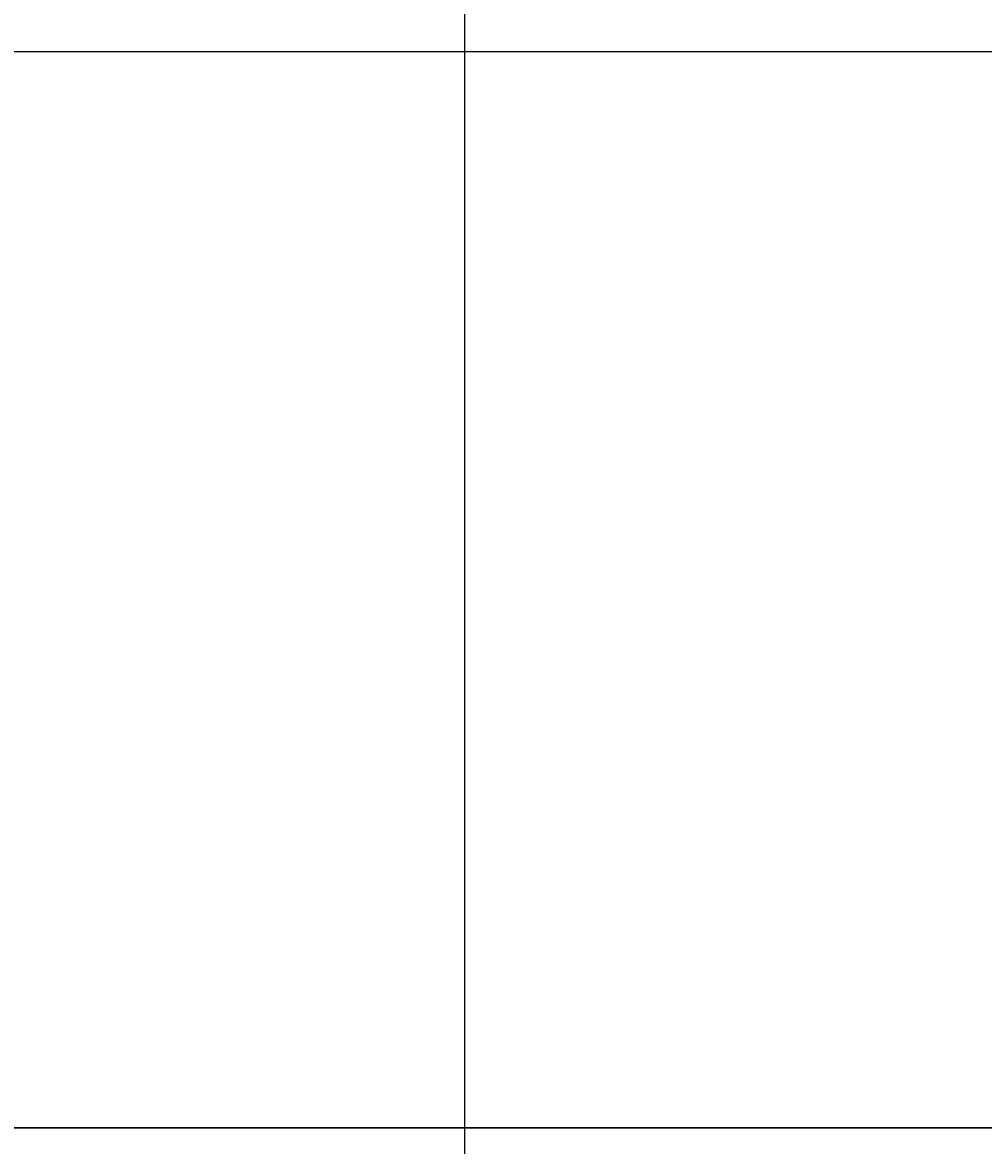
# Model space of a CAD drawing. Units: feet. Extents: x 105 to 1094, y -88 to 588.
# Tile 56 of 59: x 649 to 699, y 470 to 529. Entities that reach past the tile are written whole.
import ezdxf

# ---------------------------------------------------------------- set-up
doc = ezdxf.new("R2010")
doc.units = ezdxf.units.FT
doc.header["$MEASUREMENT"] = 0
doc.layers.add('A-ANNO-DIMS', color=2, linetype='Continuous', lineweight=18)
doc.layers.add('A-FLOR-PROJ', color=8, linetype='Continuous', lineweight=25)
doc.styles.get("Standard").update_dxf_attribs({"font": 'arial.ttf'})
doc.dimstyles.get("Standard").update_dxf_attribs({"dimtxt": 0.18, "dimasz": 0.18, "dimexe": 0.18, "dimexo": 0.0625, "dimgap": 0.09, "dimtad": 0, "dimtih": 1, "dimtoh": 1, "dimdec": 4, "dimzin": 0, "dimdsep": 46, "dimtxsty": 'Standard', "dimcen": 0.09, "dimadec": 0, "dimazin": 0, "dimtfac": 1, "dimtdec": 4, "dimtofl": 0, "dimtmove": 0, "dimatfit": 3, "dimfxl": 1, "dimtolj": 1, "dimtzin": 0, "dimarcsym": 0})

# ---------------------------------------------------------------- blocks, each defined once
blk = doc.blocks.new('*D21')
at = {"layer": 'A-ANNO-DIMS', "color": 0, "lineweight": -2, "transparency": 16777216}
for p, q in [((849.626, 543.081), (105.458, 543.081)), ((105.638, 542.901), (105.638, 250.263)), ((105.638, -42.739), (105.638, 249.899)), ((849.626, -42.919), (105.458, -42.919))]:
    blk.add_line(p, q, dxfattribs=at)
at = {"layer": 'A-ANNO-DIMS', "color": 0, "transparency": 16777216}
for points in [[(105.608, 542.901), (105.668, 542.901), (105.638, 543.081)], [(105.608, -42.739), (105.668, -42.739), (105.638, -42.919)]]:
    blk.add_solid(points, dxfattribs=at)
at = {"layer": 'Defpoints', "color": 0, "transparency": 16777216}
for p in [(105.638, 543.081), (849.688, 543.081), (849.688, -42.919)]:
    blk.add_point(p, dxfattribs=at)
at = {"layer": 'A-ANNO-DIMS', "color": 0, "transparency": 16777216, "insert": (105.638, 250.081), "char_height": 0.18, "attachment_point": 5}
blk.add_mtext('\\A1;586', dxfattribs=at)
blk = doc.blocks.new('*D30')
at = {"layer": 'A-ANNO-DIMS', "color": 0, "lineweight": -2, "transparency": 16777216}
for p, q in [((349.751, 543.081), (1093.918, 543.081)), ((1093.738, 542.901), (1093.738, 535.263)), ((1093.738, 527.261), (1093.738, 534.899)), ((349.751, 527.081), (1093.918, 527.081))]:
    blk.add_line(p, q, dxfattribs=at)
at = {"layer": 'A-ANNO-DIMS', "color": 0, "transparency": 16777216}
for points in [[(1093.708, 542.901), (1093.768, 542.901), (1093.738, 543.081)], [(1093.708, 527.261), (1093.768, 527.261), (1093.738, 527.081)]]:
    blk.add_solid(points, dxfattribs=at)
at = {"layer": 'Defpoints', "color": 0, "transparency": 16777216}
for p in [(349.688, 543.081), (349.688, 527.081), (1093.738, 527.081)]:
    blk.add_point(p, dxfattribs=at)
at = {"layer": 'A-ANNO-DIMS', "color": 0, "transparency": 16777216, "insert": (1093.738, 535.081), "char_height": 0.18, "attachment_point": 5}
blk.add_mtext('\\A1;16', dxfattribs=at)
blk = doc.blocks.new('*D31')
at = {"layer": 'A-ANNO-DIMS', "color": 0, "lineweight": -2, "transparency": 16777216}
for p, q in [((438.751, 527.081), (1093.918, 527.081)), ((1093.738, 526.901), (1093.738, 499.263)), ((1093.738, 471.261), (1093.738, 498.899)), ((438.751, 471.081), (1093.918, 471.081))]:
    blk.add_line(p, q, dxfattribs=at)
at = {"layer": 'A-ANNO-DIMS', "color": 0, "transparency": 16777216}
for points in [[(1093.708, 526.901), (1093.768, 526.901), (1093.738, 527.081)], [(1093.708, 471.261), (1093.768, 471.261), (1093.738, 471.081)]]:
    blk.add_solid(points, dxfattribs=at)
at = {"layer": 'Defpoints', "color": 0, "transparency": 16777216}
for p in [(438.688, 527.081), (1093.738, 527.081), (438.688, 471.081)]:
    blk.add_point(p, dxfattribs=at)
at = {"layer": 'A-ANNO-DIMS', "color": 0, "transparency": 16777216, "insert": (1093.738, 499.081), "char_height": 0.18, "attachment_point": 5}
blk.add_mtext('\\A1;56', dxfattribs=at)
blk = doc.blocks.new('*D41')
at = {"layer": 'A-ANNO-DIMS', "color": 0, "lineweight": -2, "transparency": 16777216}
for p, q in [((646.688, 441.144), (646.688, 588.311)), ((646.868, 588.131), (658.967, 588.131)), ((671.508, 588.131), (659.409, 588.131)), ((671.688, 441.144), (671.688, 588.311))]:
    blk.add_line(p, q, dxfattribs=at)
at = {"layer": 'A-ANNO-DIMS', "color": 0, "transparency": 16777216}
for points in [[(646.868, 588.161), (646.868, 588.101), (646.688, 588.131)], [(671.508, 588.161), (671.508, 588.101), (671.688, 588.131)]]:
    blk.add_solid(points, dxfattribs=at)
at = {"layer": 'Defpoints', "color": 0, "transparency": 16777216}
for p in [(671.688, 588.131), (646.688, 441.081), (671.688, 441.081)]:
    blk.add_point(p, dxfattribs=at)
at = {"layer": 'A-ANNO-DIMS', "color": 0, "transparency": 16777216, "insert": (659.188, 588.131), "char_height": 0.18, "attachment_point": 5}
blk.add_mtext('\\A1;25', dxfattribs=at)

msp = doc.modelspace()

# ---------------------------------------------------------------- linework, layer by layer
at = {"layer": 'A-FLOR-PROJ'}
msp.add_line((760.6883, 471.0812), (646.6883, 471.0812), dxfattribs=at)

# ---------------------------------------------------------------- dimensions: what is measured, and where the dimension line sits
at = {"layer": 'A-ANNO-DIMS'}
dim = msp.add_linear_dim(base=(671.6883, 588.1312), p1=(646.6883, 441.0812), p2=(671.6883, 441.0812), dimstyle='Standard', override={"dimdec": 0, "dimlfac": 1, "dimrnd": 0, "dimzin": 0, "dimdsep": 46, "dimlunit": 2}, dxfattribs=at)
dim.commit()
dim.dimension.update_dxf_attribs({"geometry": '*D41', "text_midpoint": (659.1883, 588.1312)})
for base, p1, p2, picture, middle in [((105.6383, 543.0812), (849.6883, -42.9188), (849.6883, 543.0812), '*D21', (105.6383, 250.0812)), ((1093.7383, 527.0812), (349.6883, 543.0812), (349.6883, 527.0812), '*D30', (1093.7383, 535.0812)), ((1093.7383, 527.0812), (438.6883, 471.0812), (438.6883, 527.0812), '*D31', (1093.7383, 499.0812))]:
    dim = msp.add_linear_dim(base=base, p1=p1, p2=p2, angle=90, dimstyle='Standard', override={"dimdec": 0, "dimlfac": 1, "dimrnd": 0, "dimzin": 0, "dimdsep": 46, "dimlunit": 2}, dxfattribs=at)
    dim.commit()
    dim.dimension.update_dxf_attribs({"geometry": picture, "text_midpoint": middle})

doc.saveas('drawing.dxf')
